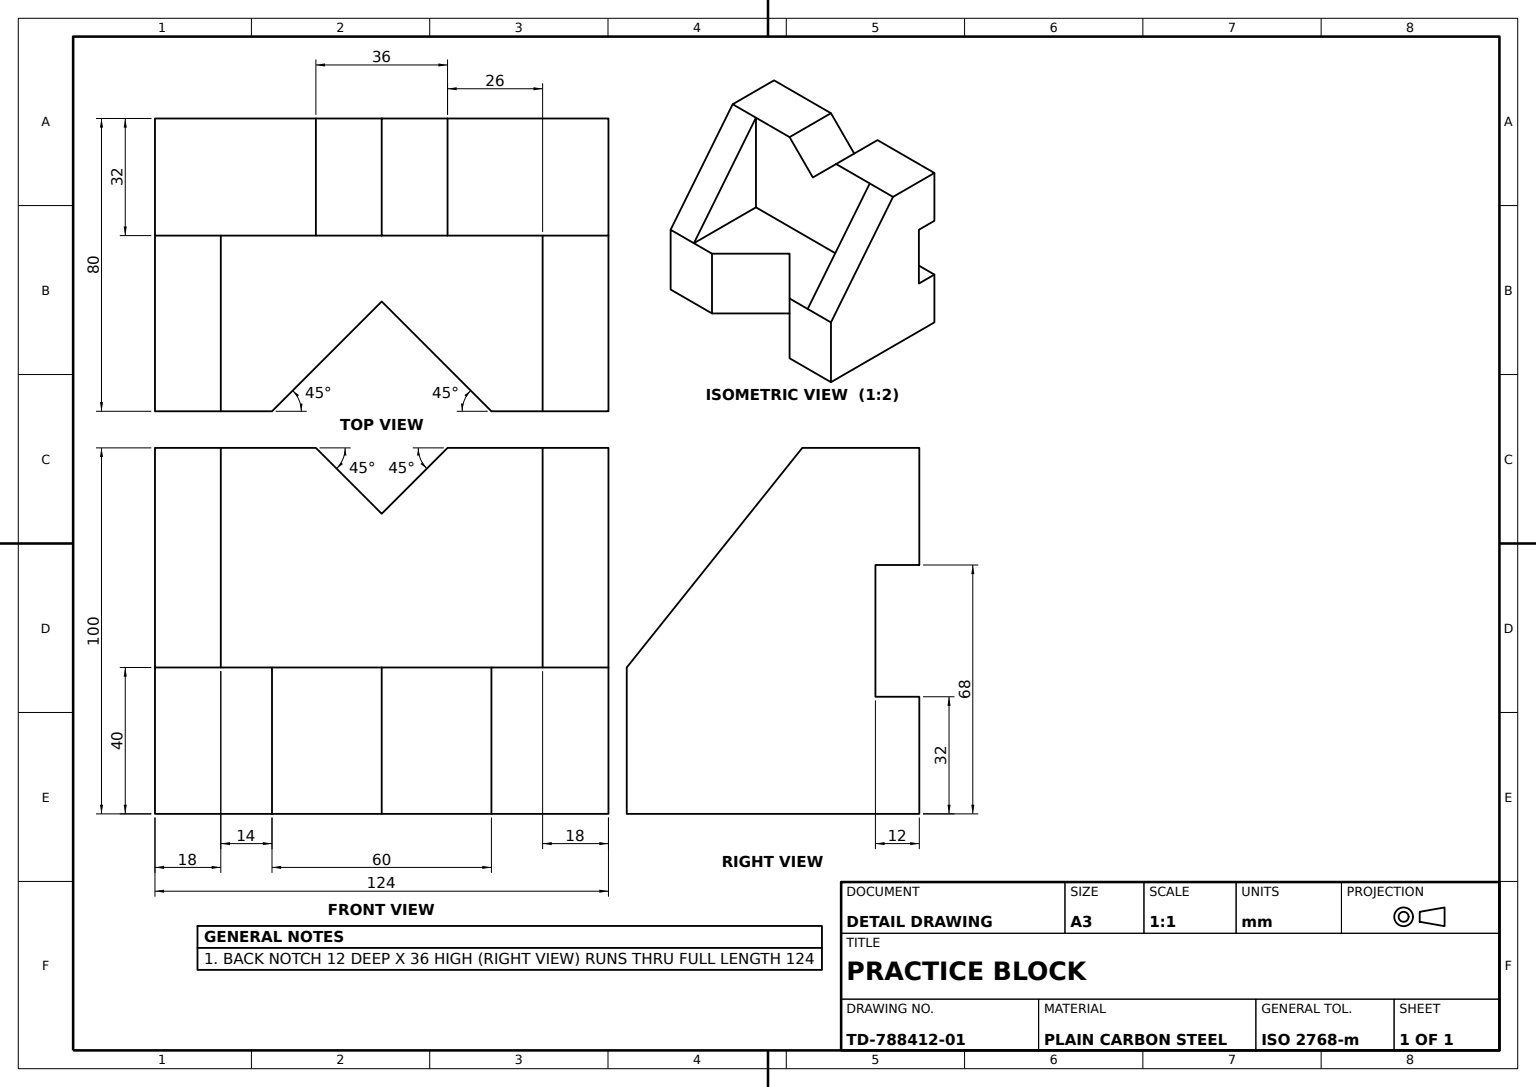
SolidWorks part; units mm, degrees
material "Plain Carbon Steel"
ref_plane "Front Plane" through (0, 0, 0) normal (0, 0, 1) x (1, 0, 0)
ref_plane "Top Plane" through (0, 0, 0) normal (0, 1, 0) x (1, 0, 0)
ref_plane "Right Plane" through (0, 0, 0) normal (1, 0, 0) x (0, 0, -1)
sketch "Base Profile Sketch" plane through (0, 0, 0) normal (0, 0, 1) x (1, 0, 0)
  line L0 (0, 0) -> (0, -100)
  line L1 (0, -100) -> (124, -100)
  line L2 (124, -100) -> (124, 0)
  line L3 (124, 0) -> (0, 0)
  dimension "D1" = 124
  dimension "D2" = 100
extrude "Base Block 32" add sketch "Base Profile Sketch" along normal blind 32
sketch "Front Notch Sketch" plane through (0, 0, 0) normal (-1, 0, 0) x (0, 0, 1)
  line L0 (32, -100) -> (0, -100) construction
  line L1 (0, 0) -> (0, -100) construction
  line L2 (0, -68) -> (12, -68)
  line L3 (12, -68) -> (12, -32)
  line L4 (12, -32) -> (0, -32)
  line L5 (0, -32) -> (0, -68)
  dimension "D1" = 12
  dimension "D2" = 32
  dimension "D3" = 68
extrude "Front Notch Cut" cut sketch "Front Notch Sketch" against normal blind 124
sketch "Upright Wall Sketch" plane through (0, -100, 0) normal (0, -1, 0) x (1, 0, 0)
  line L0 (0, 32) -> (0, 80)
  line L1 (0, 80) -> (124, 80)
  line L2 (124, 80) -> (124, 32)
  line L3 (124, 32) -> (0, 32)
  line L5 (0, 0) -> (124, 0) construction
  dimension "D1" = 80
extrude "Upright Wall 40" add sketch "Upright Wall Sketch" against normal blind 40
sketch "Wedge A Sketch" plane through (124, 0, 0) normal (1, 0, 0) x (0, 0, -1)
  line L0 (-80, -60) -> (-32, 0)
  line L1 (-32, 0) -> (-32, -60)
  line L2 (-32, -60) -> (-80, -60)
extrude "Wedge A 18" add sketch "Wedge A Sketch" against normal blind 18
sketch "Wedge B Sketch" plane through (0, 0, 0) normal (-1, 0, 0) x (0, 0, 1)
  line L0 (80, -60) -> (32, 0)
  line L1 (32, 0) -> (32, -60)
  line L2 (32, 0) -> (32, -60) construction
  line L3 (32, -60) -> (32, 0) construction
  line L4 (32, -60) -> (80, -60)
extrude "Wedge B 18" add sketch "Wedge B Sketch" against normal blind 18
sketch "V Notch Sketch" plane through (0, -60, 0) normal (0, 1, 0) x (1, 0, 0)
  line L0 (62, -80) -> (32, -80)
  line L1 (106, -80) -> (18, -80) construction
  line L2 (32, -80) -> (92, -80)
  line L4 (62, -50) -> (32, -80)
  line L5 (92, -80) -> (62, -50)
  line L6 (18, -32) -> (18, -80) construction
  line M2 (18, -80) -> (106, -80)
  dimension "D1" = 14
extrude "V Notch Cut" cut sketch "V Notch Sketch" against normal blind 40 contours L5 L4 M2
sketch "Side Slot Sketch" plane through (0, 0, 32) normal (0, 0, 1) x (1, 0, 0)
  line L0 (62, 0) -> (44, 0)
  line L1 (106, 0) -> (18, 0) construction
  line L2 (44, 0) -> (80, 0)
  line L4 (62, -18) -> (80, 0)
  line L5 (80, 0) -> (44, 0)
  line L6 (62, -18) -> (44, 0)
  line L7 (18, 0) -> (18, -60) construction
  line M4 (106, 0) -> (18, 0)
  dimension "D1" = 26
extrude "Side Slot Cut" cut sketch "Side Slot Sketch" against normal blind 40 contours L6 L4 M4
